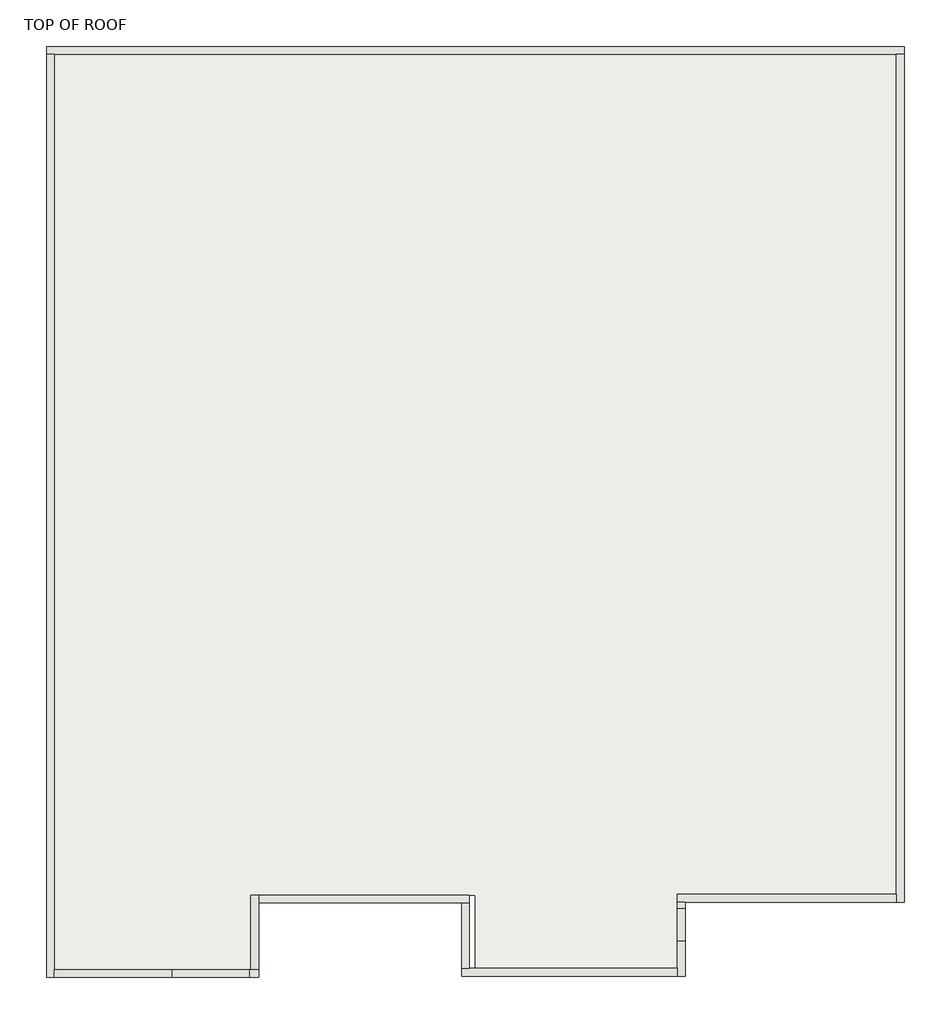
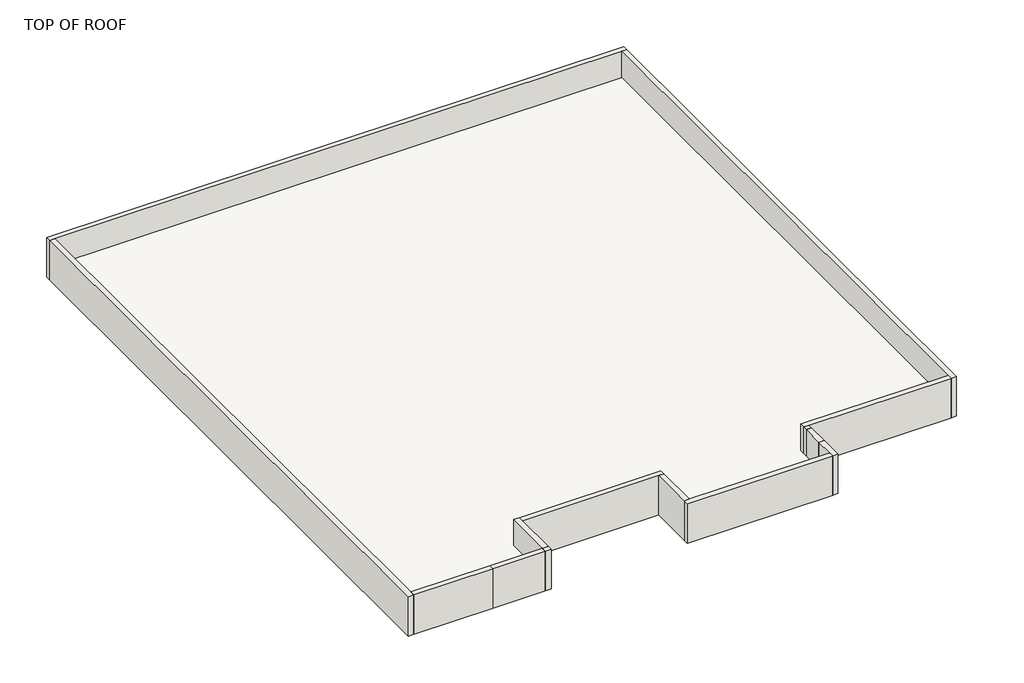
# One storey: 14 walls, 1 roof.
"""IFC4 building model written with IfcOpenShell, lengths in millimetres."""

from ifc_helpers import new_model, si_unit, frame, origin, place, context, project, spatial, polyline, outline, extrude, faceted_brep, element, save

model = new_model("IFC4")

# Units and contexts
model_context = context("Model", 3, world=origin())
ifc_project = project(units=[si_unit("LENGTHUNIT", "METRE", prefix="MILLI")], contexts=[model_context])

# Site, building, storey
site = spatial("IfcSite", under=ifc_project)
building = spatial("IfcBuilding", under=site)
storey = spatial("IfcBuildingStorey", under=building, Name="TOP OF ROOF", Elevation=6400.8)

# Roof
placement = place(None, origin())
element("IfcRoof", 1, ObjectType="Generic - 12\"", at=placement, inside=storey, context=model_context, shape_type="SweptSolid", body=[
    extrude(outline(polyline([(-18148.9007021, -5315.3090801), (-18148.9007021, 8172.0909199), (-5742.8860997, 8172.0909199), (-5742.8860997, -4215.4340831), (-8943.2860997, -4215.4340831), (-8943.2860997, -5316.3582515), (-11945.8934009, -5316.3582515), (-11945.8934009, -4215.4340831), (-15253.300702, -4215.4340831), (-15253.300702, -5315.3090801), (-18148.9007021, -5315.3090801)])), frame((0.0, 0.0, 6400.8), z_axis=(0.0, 0.0, 1.0), x_axis=(1.0, 0.0, 0.0)), (0.0, 0.0, 1.0), 304.8),
])

# Walls
element("IfcWall", 2, at=placement, inside=storey, context=model_context, shape_type="Brep", body=[
    faceted_brep([(-18263.2007021, 8172.0909199, 6400.8), (-18148.9007021, 8172.0909199, 6400.8), (-5742.8860997, 8172.0909199, 6400.8), (-5628.5860997, 8172.0909199, 6400.8), (-5628.5860997, 8172.0909199, 7315.2), (-5742.8860997, 8172.0909199, 7315.2), (-18148.9007021, 8172.0909199, 7315.2), (-18263.2007021, 8172.0909199, 7315.2), (-18263.2007021, 8286.3909199, 6400.8), (-18263.2007021, 8286.3909199, 7315.2), (-5628.5860997, 8286.3909199, 7315.2), (-5628.5860997, 8286.3909199, 6400.8)], [[[0, 1, 2, 3, 4, 5, 6, 7]], [[8, 9, 10, 11]], [[3, 2, 1, 0, 8, 11]], [[7, 6, 5, 4, 10, 9]], [[4, 3, 11, 10]], [[0, 7, 9, 8]]]),
])
element("IfcWall", 3, at=placement, inside=storey, context=model_context, shape_type="Brep", body=[
    faceted_brep([(-5742.8860997, 8172.0909199, 6400.8), (-5742.8860997, -4204.0590801, 6400.8), (-5742.8860997, -4318.3590801, 6400.8), (-5742.8860997, -4318.3590801, 7315.2), (-5742.8860997, -4204.0590801, 7315.2), (-5742.8860997, 8172.0909199, 7315.2), (-5628.5860997, 8172.0909199, 6400.8), (-5628.5860997, 8172.0909199, 7315.2), (-5628.5860997, -4318.3590801, 7315.2), (-5628.5860997, -4318.3590801, 6400.8)], [[[0, 1, 2, 3, 4, 5]], [[6, 7, 8, 9]], [[2, 1, 0, 6, 9]], [[5, 4, 3, 8, 7]], [[0, 5, 7, 6]], [[3, 2, 9, 8]]]),
])
element("IfcWall", 4, at=placement, inside=storey, context=model_context, shape_type="Brep", body=[
    faceted_brep([(-5742.8860997, -4204.0590801, 6400.8), (-8968.6860997, -4204.0590801, 6400.8), (-8968.6860997, -4204.0590801, 7315.2), (-5742.8860997, -4204.0590801, 7315.2), (-5742.8860997, -4318.3590801, 6400.8), (-5742.8860997, -4318.3590801, 7315.2), (-8854.3860997, -4318.3590801, 7315.2), (-8968.6860997, -4318.3590801, 7315.2), (-8968.6860997, -4318.3590801, 6400.8), (-8854.3860997, -4318.3590801, 6400.8)], [[[0, 1, 2, 3]], [[4, 5, 6, 7, 8, 9]], [[1, 0, 4, 9, 8]], [[3, 2, 7, 6, 5]], [[0, 3, 5, 4]], [[2, 1, 8, 7]]]),
])
element("IfcWall", 5, at=placement, inside=storey, context=model_context, shape_type="SweptSolid", body=[
    extrude(outline(polyline([(-8968.6860997, -4413.6090801), (-8968.6860997, -4318.3590801), (-8854.3860997, -4318.3590801), (-8854.3860997, -4413.6090801), (-8968.6860997, -4413.6090801)])), frame((0.0, 0.0, 6400.8), z_axis=(0.0, 0.0, 1.0), x_axis=(1.0, 0.0, 0.0)), (0.0, 0.0, 1.0), 914.4),
])
element("IfcWall", 6, at=placement, inside=storey, context=model_context, shape_type="Brep", body=[
    faceted_brep([(-8968.6860997, -5296.2590801, 6400.8), (-12034.7934009, -5296.2590801, 6400.8), (-12149.0934009, -5296.2590801, 6400.8), (-12149.0934009, -5296.2590801, 7315.2), (-12034.7934009, -5296.2590801, 7315.2), (-8968.6860997, -5296.2590801, 7315.2), (-8968.6860997, -5410.5590801, 6400.8), (-8968.6860997, -5410.5590801, 7315.2), (-12149.0934009, -5410.5590801, 7315.2), (-12149.0934009, -5410.5590801, 6400.8)], [[[0, 1, 2, 3, 4, 5]], [[6, 7, 8, 9]], [[2, 1, 0, 6, 9]], [[5, 4, 3, 8, 7]], [[0, 5, 7, 6]], [[3, 2, 9, 8]]]),
])
element("IfcWall", 7, at=placement, inside=storey, context=model_context, shape_type="Brep", body=[
    faceted_brep([(-18263.2007021, 8172.0909199, 6400.8), (-18263.2007021, -5429.6090801, 6400.8), (-18263.2007021, -5429.6090801, 7315.2), (-18263.2007021, 8172.0909199, 7315.2), (-18148.9007021, 8172.0909199, 6400.8), (-18148.9007021, 8172.0909199, 7315.2), (-18148.9007021, -5315.3090801, 7315.2), (-18148.9007021, -5429.6090801, 7315.2), (-18148.9007021, -5429.6090801, 6400.8), (-18148.9007021, -5315.3090801, 6400.8)], [[[0, 1, 2, 3]], [[4, 5, 6, 7, 8, 9]], [[1, 0, 4, 9, 8]], [[3, 2, 7, 6, 5]], [[0, 3, 5, 4]], [[2, 1, 8, 7]]]),
])
element("IfcWall", 8, at=placement, inside=storey, context=model_context, shape_type="SweptSolid", body=[
    extrude(outline(polyline([(-16415.350702, -5429.6090801), (-18148.9007021, -5429.6090801), (-18148.9007021, -5315.3090801), (-16415.350702, -5315.3090801), (-16415.350702, -5429.6090801)])), frame((0.0, 0.0, 6400.8), z_axis=(0.0, 0.0, 1.0), x_axis=(1.0, 0.0, 0.0)), (0.0, 0.0, 1.0), 914.4),
])
element("IfcWall", 9, at=placement, inside=storey, context=model_context, shape_type="Brep", body=[
    faceted_brep([(-15139.000702, -5315.3090801, 6400.8), (-15139.000702, -4329.734083, 6400.8), (-15139.000702, -4215.434083, 6400.8), (-15139.000702, -4215.434083, 7315.2), (-15139.000702, -4329.734083, 7315.2), (-15139.000702, -5315.3090801, 7315.2), (-15253.300702, -5315.3090801, 6400.8), (-15253.300702, -5315.3090801, 7315.2), (-15253.300702, -4215.434083, 7315.2), (-15253.300702, -4215.434083, 6400.8)], [[[0, 1, 2, 3, 4, 5]], [[6, 7, 8, 9]], [[2, 1, 0, 6, 9]], [[5, 4, 3, 8, 7]], [[0, 5, 7, 6]], [[3, 2, 9, 8]]]),
])
element("IfcWall", 10, at=placement, inside=storey, context=model_context, shape_type="Brep", body=[
    faceted_brep([(-15139.000702, -4329.734083, 6400.8), (-12149.0934009, -4329.734083, 6400.8), (-12034.7934009, -4329.734083, 6400.8), (-12034.7934009, -4329.734083, 7315.2), (-12149.0934009, -4329.734083, 7315.2), (-15139.000702, -4329.734083, 7315.2), (-15139.000702, -4215.434083, 6400.8), (-15139.000702, -4215.434083, 7315.2), (-12034.7934009, -4215.434083, 7315.2), (-12034.7934009, -4215.434083, 6400.8)], [[[0, 1, 2, 3, 4, 5]], [[6, 7, 8, 9]], [[2, 1, 0, 6, 9]], [[5, 4, 3, 8, 7]], [[0, 5, 7, 6]], [[3, 2, 9, 8]]]),
])
element("IfcWall", 11, at=placement, inside=storey, context=model_context, shape_type="SweptSolid", body=[
    extrude(outline(polyline([(-12149.0934009, -5296.2590801), (-12149.0934009, -4329.734083), (-12034.7934009, -4329.734083), (-12034.7934009, -5296.2590801), (-12149.0934009, -5296.2590801)])), frame((0.0, 0.0, 6400.8), z_axis=(0.0, 0.0, 1.0), x_axis=(1.0, 0.0, 0.0)), (0.0, 0.0, 1.0), 914.4),
])
element("IfcWall", 12, at=placement, inside=storey, context=model_context, shape_type="Brep", body=[
    faceted_brep([(-15272.350702, -5429.6090801, 6400.8), (-15139.000702, -5429.6090801, 6400.8), (-15139.000702, -5429.6090801, 7315.2), (-15272.350702, -5429.6090801, 7315.2), (-15272.350702, -5315.3090801, 6400.8), (-15272.350702, -5315.3090801, 7315.2), (-15253.300702, -5315.3090801, 7315.2), (-15139.000702, -5315.3090801, 7315.2), (-15139.000702, -5315.3090801, 6400.8), (-15253.300702, -5315.3090801, 6400.8)], [[[0, 1, 2, 3]], [[4, 5, 6, 7, 8, 9]], [[1, 0, 4, 9, 8]], [[3, 2, 7, 6, 5]], [[0, 3, 5, 4]], [[2, 1, 8, 7]]]),
])
element("IfcWall", 13, at=placement, inside=storey, context=model_context, shape_type="SweptSolid", body=[
    extrude(outline(polyline([(-15272.350702, -5429.6090801), (-16415.350702, -5429.6090801), (-16415.350702, -5315.3090801), (-15272.350702, -5315.3090801), (-15272.350702, -5429.6090801)])), frame((0.0, 0.0, 6400.8), z_axis=(0.0, 0.0, 1.0), x_axis=(1.0, 0.0, 0.0)), (0.0, 0.0, 1.0), 914.4),
])
element("IfcWall", 14, at=placement, inside=storey, context=model_context, shape_type="Brep", body=[
    faceted_brep([(-8968.6860997, -4896.2090801, 6400.8), (-8968.6860997, -5296.2590801, 6400.8), (-8968.6860997, -5410.5590801, 6400.8), (-8968.6860997, -5410.5590801, 7315.2), (-8968.6860997, -5296.2590801, 7315.2), (-8968.6860997, -4896.2090801, 7315.2), (-8854.3860997, -4896.2090801, 6400.8), (-8854.3860997, -4896.2090801, 7315.2), (-8854.3860997, -5410.5590801, 7315.2), (-8854.3860997, -5410.5590801, 6400.8)], [[[0, 1, 2, 3, 4, 5]], [[6, 7, 8, 9]], [[2, 1, 0, 6, 9]], [[5, 4, 3, 8, 7]], [[0, 5, 7, 6]], [[3, 2, 9, 8]]]),
])
element("IfcWall", 15, at=placement, inside=storey, context=model_context, shape_type="SweptSolid", body=[
    extrude(outline(polyline([(-8968.6860997, -4896.2090801), (-8968.6860997, -4413.6090801), (-8854.3860997, -4413.6090801), (-8854.3860997, -4896.2090801), (-8968.6860997, -4896.2090801)])), frame((0.0, 0.0, 6400.8), z_axis=(0.0, 0.0, 1.0), x_axis=(1.0, 0.0, 0.0)), (0.0, 0.0, 1.0), 914.4),
])

save(model, "model.ifc")

# Revit data of these elements
# Type "Generic - 12\""
#   Assembly Code = "B1020"
#   Layers, outside or top first: 1' - 0" no material (function 1)
# Type
#   Assembly Code = "B2010"
# Element 1 (IfcRoof, "Generic - 12\"")
#   built-in parameter 1001705 = 22 (stored number, unit not read)
#   built-in parameter 1001710 = 33615
#   Phase Created = New Construction
#   Materials on its faces: "Default Roof"
# Elements 2, 3, 4, 10 (IfcWall)
#   Top Offset = 0' - 0"
#   Base Offset = 0' - 0"
#   Unconnected Height = 3' - 0"
#   wall height = 3' - 0"
#   Phase Created = New Construction
#   Base Constraint = TOP OF ROOF
#   Materials on its faces: "red brown cladding"
# Elements 5, 6, 9, 11, 14, 15 (IfcWall)
#   Top Offset = 0' - 0"
#   Base Offset = 0' - 0"
#   Unconnected Height = 3' - 0"
#   wall height = 3' - 0"
#   Phase Created = New Construction
#   Base Constraint = TOP OF ROOF
# Elements 7, 8, 12, 13 (IfcWall)
#   Top Offset = 0' - 0"
#   Base Offset = 0' - 0"
#   Unconnected Height = 3' - 0"
#   wall height = 3' - 0"
#   Phase Created = New Construction
#   Base Constraint = TOP OF ROOF
#   Materials on its faces: "Clad - White"
# Materials
#   "Default Roof": colour RGB 88 101 114, transparency 0, Cost = 0
#   "red brown cladding": class "Generic", colour RGB 151 67 57, transparency 0, Cost = 0
#   "Clad - White": class "Wood", colour RGB 242 242 238, transparency 0, Cost = 0
